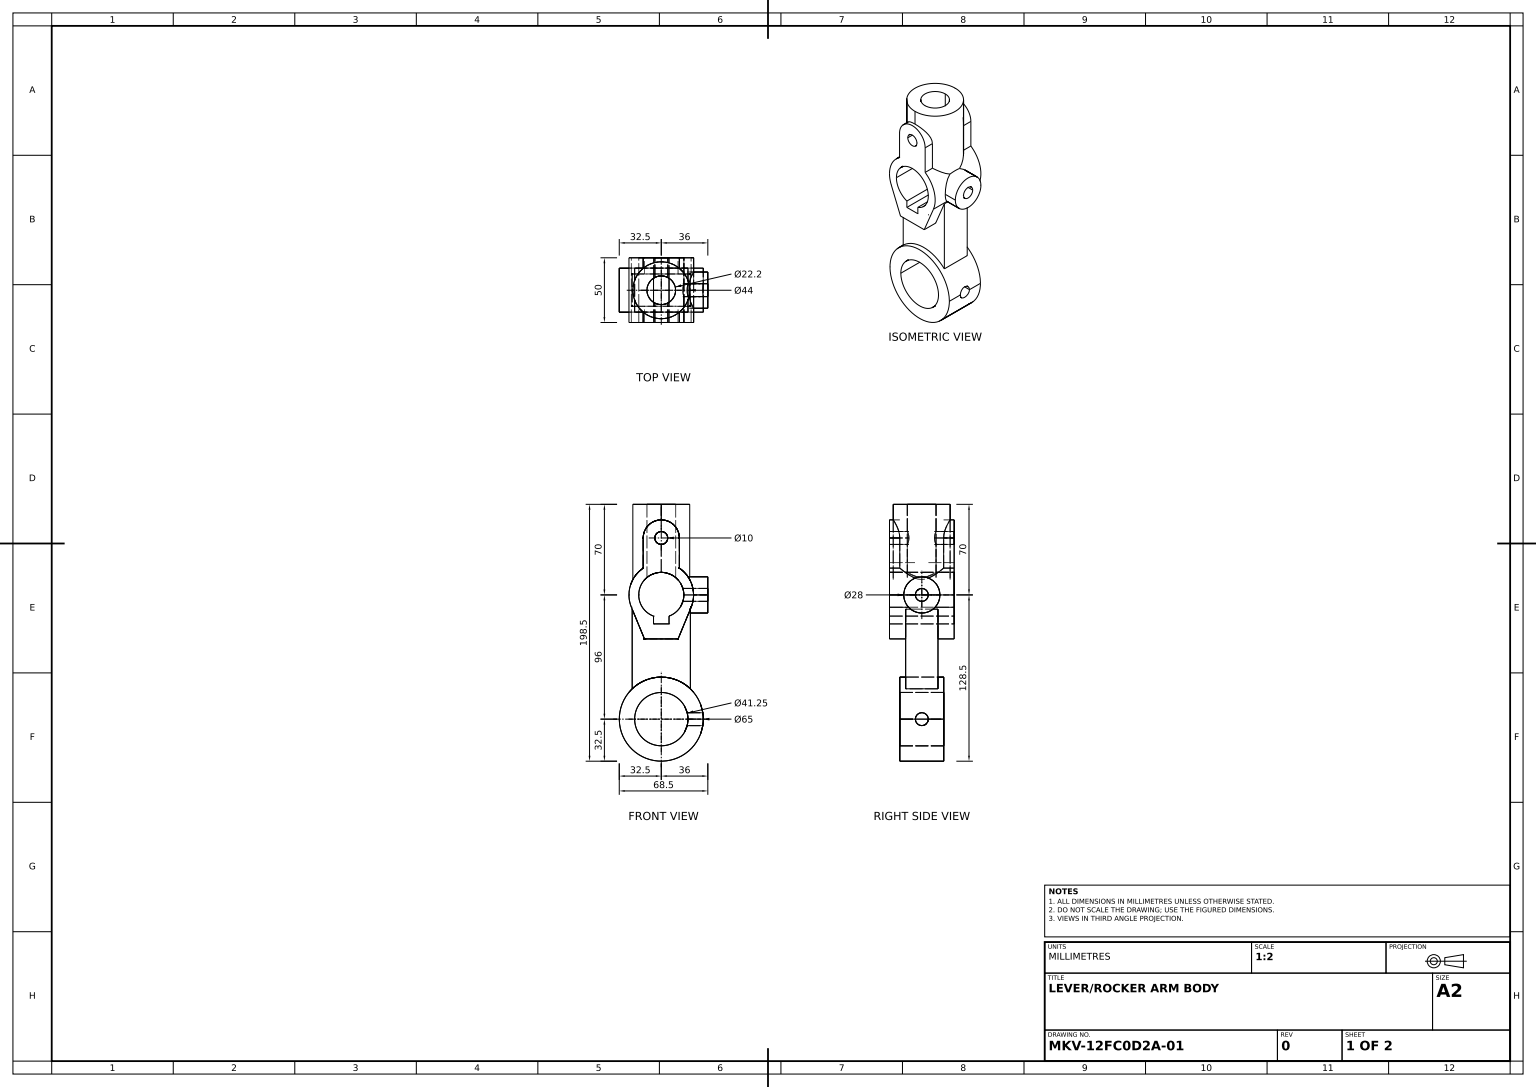
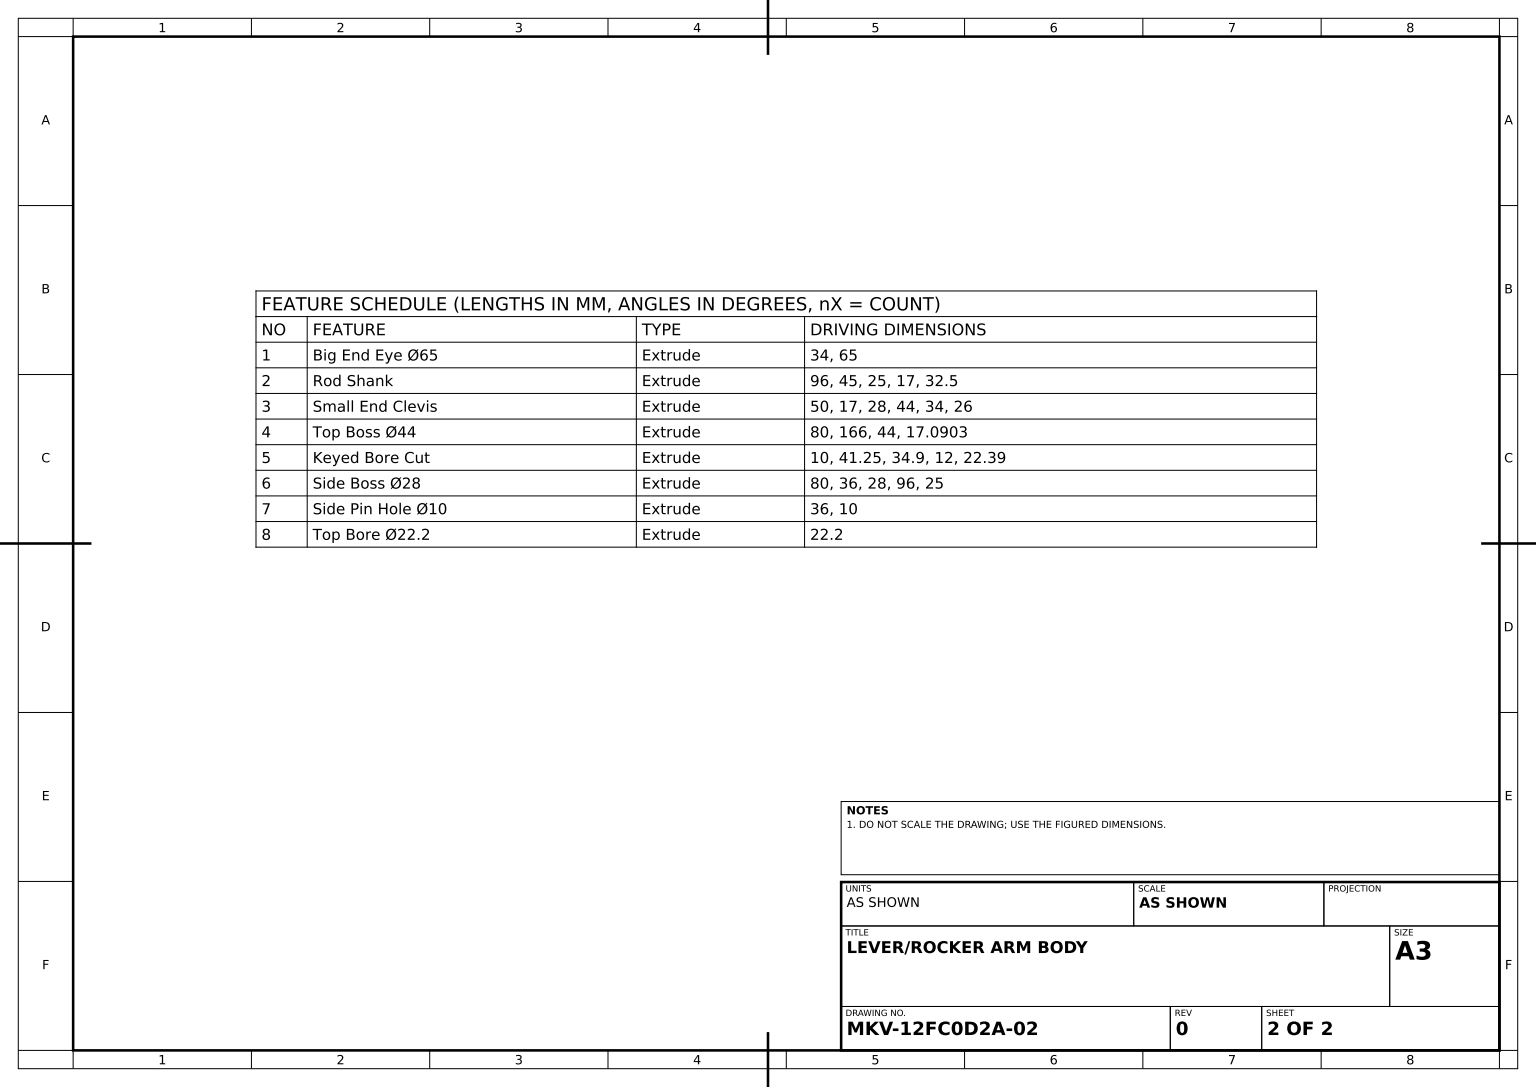
from build123d import *

# Parameters (mm, degrees)
BIG_END_EYE_SKETCH_R     = 32.5
BIG_END_EYE_65_DEPTH     = 34
ROD_SHANK_SKETCH_W       = 45
ROD_SHANK_SKETCH_H       = 25
ROD_SHANK_DEPTH          = 96
SMALL_START              = 17
SMALL_END_CLEVIS_DEPTH   = 25
TOP_START                = 166
TOP_BOSS_SKETCH_R        = 22
TOP_BOSS_44_DEPTH        = 80
KEYED_BORE_SKETCH_R      = 20.625
KEYED_BORE_SKETCH_R_2    = 5
KEYED_BORE_CUT_DEPTH     = 177.386649277
SIDE_START               = 21.354774
SIDE_BOSS_SKETCH_R       = 14
SIDE_BOSS_28_DEPTH       = 14.645226
SIDE_PIN_HOLE_SKETCH_R   = 5
SIDE_PIN_HOLE_10_DEPTH   = 36
TOP_BORE_22_2_REACH      = 208.064
TOP_BORE_22_2_END_RADIUS = 17.45
TOP_BORE_SKETCH_R        = 11.1


with BuildPart() as part:
    # Big End Eye Sketch → Big End Eye Ø65 (new body)
    with BuildSketch(Plane.XY):
        Circle(BIG_END_EYE_SKETCH_R)
    extrude(amount=BIG_END_EYE_65_DEPTH)

    # Rod Shank Sketch → Rod Shank (add)
    with BuildSketch(Plane(origin=(0, 0, 0), x_dir=(1, 0, 0), z_dir=(0, 1, 0))):
        with Locations((0, -17)):
            Rectangle(ROD_SHANK_SKETCH_W, ROD_SHANK_SKETCH_H)
    extrude(amount=ROD_SHANK_DEPTH)

    # Small End Clevis Sketch → Small End Clevis (add, symmetric)
    with BuildSketch(Plane.XY.offset(SMALL_START)):
        with BuildLine():
            Line((-14, 140), (-14, 116.712315177))
            ThreePointArc((-14, 116.712315177), (-23.9398404, 103.203057798), (-23.104819731, 86.451842838))
            Line((-23.104819731, 86.451842838), (-13, 62))
            Line((-13, 62), (13, 62))
            Line((13, 62), (23.104819731, 86.451842838))
            ThreePointArc((23.104819731, 86.451842838), (23.9398404, 103.203057798), (14, 116.712315177))
            Line((14, 116.712315177), (14, 140))
            ThreePointArc((14, 140), (0, 154), (-14, 140))
        make_face()
    extrude(amount=SMALL_END_CLEVIS_DEPTH, both=True)

    # Top Boss Sketch → Top Boss Ø44 (add)
    with BuildSketch(Plane(origin=(0, 0, 0), x_dir=(1, 0, 0), z_dir=(0, 1, 0)).offset(TOP_START)):
        with Locations(Location((0, -17.090316824, 0), (0, 0, 270))):
            Circle(TOP_BOSS_SKETCH_R)
    extrude(amount=-TOP_BOSS_44_DEPTH)

    # Keyed Bore Sketch → Keyed Bore Cut (cut, through all)
    with BuildSketch(Plane(origin=(0, 0, -8), x_dir=(-1, 0, 0), z_dir=(0, 0, -1))):
        with Locations(Location((0, 0, 0), (0, 0, 180))):
            Circle(KEYED_BORE_SKETCH_R)
        with Locations((0, 140)):
            Circle(KEYED_BORE_SKETCH_R_2)
        with BuildLine():
            Line((-6, 79.613954107), (-6, 73.61))
            Line((-6, 73.61), (6, 73.61))
            Line((6, 73.61), (6, 79.613954107))
            ThreePointArc((6, 79.613954107), (0, 113.45), (-6, 79.613954107))
        make_face()
    extrude(amount=-KEYED_BORE_CUT_DEPTH, mode=Mode.SUBTRACT)

    # Side Boss Sketch → Side Boss Ø28 (add)
    with BuildSketch(Plane(origin=(0, 0, 0), x_dir=(0, 0, -1), z_dir=(1, 0, 0)).offset(SIDE_START)):
        with Locations((-17, 96)):
            Circle(SIDE_BOSS_SKETCH_R)
    extrude(amount=SIDE_BOSS_28_DEPTH)

    # Side Pin Hole Sketch → Side Pin Hole Ø10 (cut)
    with BuildSketch(Plane(origin=(36, 0, 0), x_dir=(0, 0, -1), z_dir=(1, 0, 0))):
        with Locations((-17, 96)):
            Circle(SIDE_PIN_HOLE_SKETCH_R)
        with Locations((-17, 0)):
            Circle(SIDE_PIN_HOLE_SKETCH_R)
    extrude(amount=-SIDE_PIN_HOLE_10_DEPTH, mode=Mode.SUBTRACT)

    # Top Bore Ø22.2: up to this cylinder (the profile starts outside it)
    top_bore_22_2_end = Plane(origin=(0, 96, 17.090317), z_dir=(0, 0, -1)) * Cylinder(TOP_BORE_22_2_END_RADIUS, 452.028, mode=Mode.PRIVATE)
    # Top Bore Sketch → Top Bore Ø22.2 (cut, up to the surface)
    with BuildSketch(Plane(origin=(0, 166, 0), x_dir=(1, 0, 0), z_dir=(0, 1, 0)), mode=Mode.PRIVATE) as top_bore_22_2_sk1:
        with Locations(Location((0, -17.090316824, 0), (0, 0, 270))):
            Circle(TOP_BORE_SKETCH_R)
    top_bore_22_2_tool1 = extrude(top_bore_22_2_sk1.sketch, amount=-TOP_BORE_22_2_REACH, mode=Mode.PRIVATE) - top_bore_22_2_end
    add(top_bore_22_2_tool1.solids().sort_by_distance((0, 166, 17.090317))[0], mode=Mode.SUBTRACT)


solid = part.part
